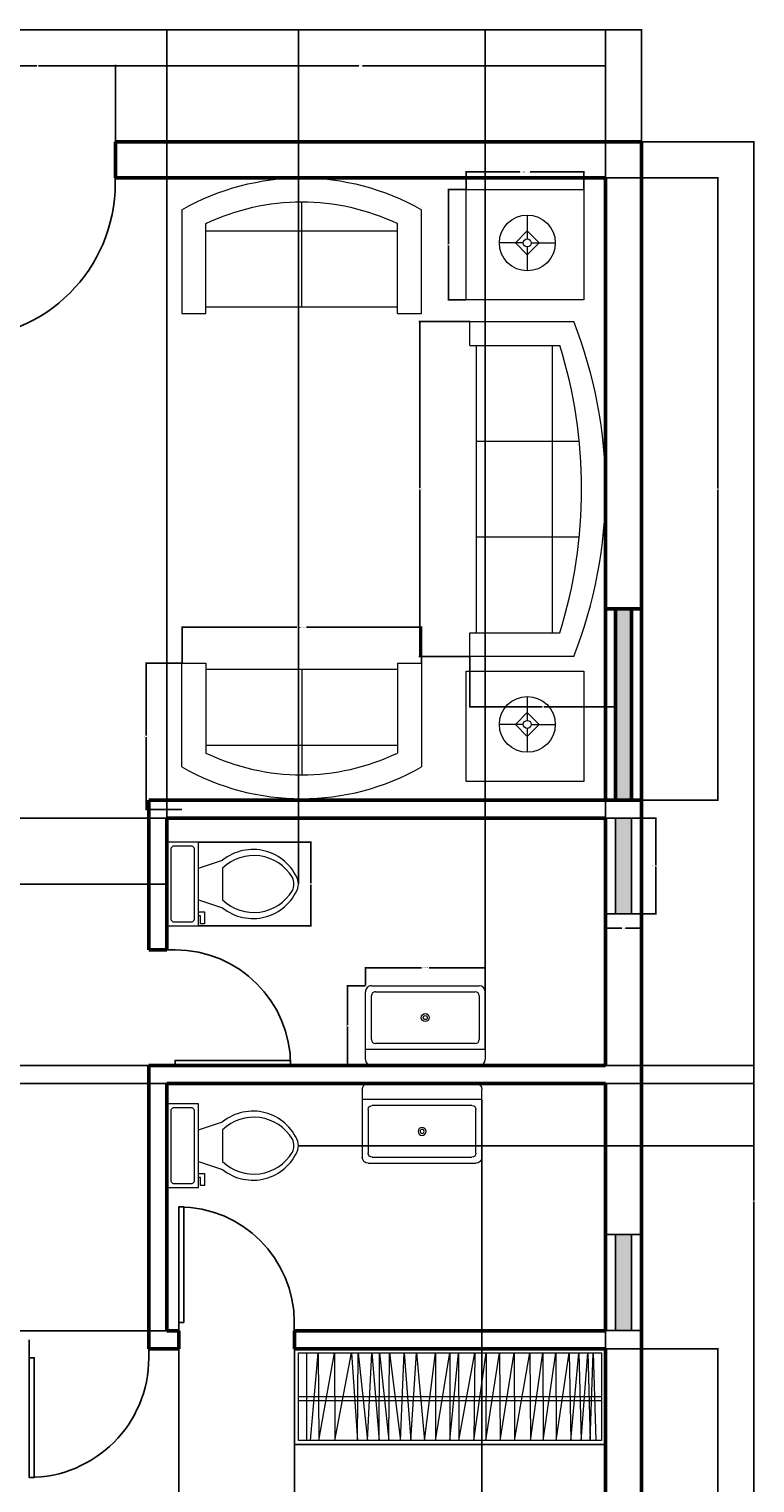
# Model space of a CAD drawing. Units: inches. Extents: x 1974 to 2406, y 1583 to 2170.
# Tile 6 of 6: x 2224 to 2406, y 1806 to 2170. Entities that reach past the tile are written whole.
import ezdxf

# ---------------------------------------------------------------- set-up
doc = ezdxf.new("R2010")
doc.units = ezdxf.units.IN
for name, color, linetype, lineweight in [('A-ANNO-DIMS', 2, 'Continuous', 18), ('A-FLOR-FIXT', 3, 'Continuous', 18), ('A-FURN', 3, 'Continuous', 18), ('A-GLAZ', 4, 'Continuous', 25), ('door', 60, 'Continuous', 25), ('wall', 240, 'Continuous', 50)]:
    doc.layers.add(name, color=color, linetype=linetype, lineweight=lineweight)
doc.layers.add('A-FLOR-CASE', color=40, linetype='Continuous', lineweight=18, true_color=0xf8d731)
doc.styles.get("Standard").update_dxf_attribs({"font": 'arial.ttf'})
doc.dimstyles.get("Standard").update_dxf_attribs({"dimtxt": 0.18, "dimasz": 0.18, "dimexe": 0.18, "dimexo": 0.0625, "dimgap": 0.09, "dimtad": 0, "dimtih": 1, "dimtoh": 1, "dimdec": 4, "dimzin": 0, "dimdsep": 46, "dimtxsty": 'Standard', "dimcen": 0.09, "dimadec": 0, "dimazin": 0, "dimtfac": 1, "dimtdec": 4, "dimtofl": 0, "dimtmove": 0, "dimatfit": 3, "dimfxl": 1, "dimtolj": 1, "dimtzin": 0, "dimarcsym": 0})

# ---------------------------------------------------------------- blocks, each defined once
blk = doc.blocks.new('*U2')
for p, q in [((0, 0), (0, -6)), ((40, 0), (40, -6))]:
    blk.add_line(p, q)
blk.add_lwpolyline([(0, 0), (0, 40), (1.75, 40), (1.75, 0)], close=True)
blk.add_arc((0, 0), 40, 0, 90)
blk = doc.blocks.new('b')
at = {"layer": 'wall'}
h = blk.add_hatch(color=256, dxfattribs=at)
h.dxf.hatch_style = 1
h.paths.add_polyline_path([(6.5, 0), (2.5, 0), (2.5, -48), (6.5, -48)])
for p, q in [((2.5, 0), (2.5, -48)), ((6.5, 0), (6.5, -48))]:
    blk.add_line(p, q, dxfattribs=at)
blk.add_lwpolyline([(0, -48), (9, -48), (9, 0), (0, 0)], close=True, dxfattribs=at)
blk = doc.blocks.new('*U7')
for p, q in [((9.5, -6), (9.5, -2)), ((-10, -8.5), (-8, -8.5)), ((-10, -9.5), (-10, -8.5)), ((-7, -9.5), (-10, -9.5)), ((-8, -8.5), (-8, -8)), ((-7, -8), (-7, -9.5)), ((-4, -8), (-6, -14)), ((4, -8), (6, -14)), ((4, -14), (-4, -14))]:
    blk.add_line(p, q)
blk.add_lwpolyline([(10.5, -8), (10.5, 0), (-10.5, 0), (-10.5, -8)], close=True)
for points in [[(-9.5, -2), (-9.5, -6)], [(8.5, -1), (-8.5, -1)], [(-8.5, -7), (8.5, -7)]]:
    blk.add_lwpolyline(points)
for centre, radius, start, end in [((-8.62, -1.88), 0.884, 81.8699, 188.1301), ((8.62, -1.88), 0.884, 351.8699, 98.1301), ((-8.62, -6.12), 0.884, 171.8699, 278.1301), ((8.62, -6.12), 0.884, 261.8699, 8.1301), ((3.52, -21.58), 12.17, 141.4691, 247.9714), ((4.2, -21.82), 11.33, 136.3677, 238.9468), ((-3.52, -21.58), 12.17, 292.0284, 38.5307), ((-4.2, -21.82), 11.33, 301.053, 43.6321), ((0, -27.88), 4, 245.7318, 294.2682), ((0, -29), 4, 254.8605, 285.1395)]:
    blk.add_arc(centre, radius, start, end)
blk = doc.blocks.new('Sink-single - 30 in top')
blk.add_line((-15, -3.999996), (15, -3.999996))
for points in [[(-13.5, 0), (13.5, 0)], [(-15, -18.499996), (-15, -1.5)], [(15, -1.5), (15, -18.499996)], [(-13.5, -17.499996), (-13.5, -6.499996)], [(-12.5, -5.499996), (12.5, -5.499996)], [(13.5, -6.499996), (13.5, -17.499996)], [(13.5, -19.999996), (-13.5, -19.999996)], [(12.5, -18.499996), (-12.5, -18.499996)]]:
    blk.add_lwpolyline(points)
for radius in [1, 0.5]:
    blk.add_circle((0, -11.999996), radius)
for centre, radius, start, end in [((-13.5, -1.5), 1.5, 90, 180), ((13.5, -1.5), 1.5, 0, 90), ((-12.5, -6.499996), 1, 90, 180), ((12.5, -6.499996), 1, 0, 90), ((-12.5, -17.499996), 1, 180, 270), ((12.5, -17.499996), 1, 270, 0), ((-13.5, -18.499996), 1.5, 180, 270), ((13.5, -18.499996), 1.5, 270, 0)]:
    blk.add_arc(centre, radius, start, end)
blk = doc.blocks.new('Sofa - Roundback 7 ft.')
for p, q in [((-12.00002, -32.4421), (-12.00003, -6.5971)), ((11.99997, -32.4421), (11.99998, -6.5971)), ((-36.000027, -34), (-36.000027, -11.4696)), ((-35.999844, -13.3819), (35.9998, -13.3819)), ((35.99998, -34), (35.99998, -11.4696)), ((-36.000027, -32.4421), (35.99998, -32.4421))]:
    blk.add_line(p, q)
for points in [[(-36.000027, -34), (-42.000027, -34), (-42.000027, -8)], [(41.99998, -8), (41.99998, -34), (35.99998, -34)]]:
    blk.add_lwpolyline(points)
for centre, radius, start, end in [((0, -114.25), 114.25, 68.43141, 111.5686), ((-0.00001, -127.1968), 121.1968, 72.72033, 107.2797)]:
    blk.add_arc(centre, radius, start, end)
blk = doc.blocks.new('Sofa - Roundback Loveseat 5 ft.')
for p, q in [((0, -32.44198), (0, -5.99998)), ((-24, -33.99998), (-24, -11.46958)), ((-23.9998, -13.38178), (23.99986, -13.38178)), ((24.00004, -33.99998), (24.00004, -11.46958)), ((-24, -32.44198), (24.00004, -32.44198))]:
    blk.add_line(p, q)
for points in [[(-24, -33.99998), (-30, -33.99998), (-30, -7.99998)], [(30.00004, -7.99998), (30.00004, -33.99998), (24.00004, -33.99998)]]:
    blk.add_lwpolyline(points)
for centre, radius, start, end in [((0, -60.24998), 60.24998, 60.13715, 119.8628), ((0, -61.38438), 55.38444, 64.32083, 115.6792)]:
    blk.add_arc(centre, radius, start, end)
blk = doc.blocks.new('Lamp - Table')
for p, q in [((0, 7), (0, 1)), ((-1, 0), (-7, 0)), ((0, 3), (-3, 0)), ((-3, 0), (0, -3)), ((3, 0), (0, 3)), ((0, -3), (3, 0)), ((1, 0), (7, 0)), ((0, -1), (0, -7))]:
    blk.add_line(p, q)
for radius in [7, 1]:
    blk.add_circle((0, 0), radius)
blk = doc.blocks.new('WINDOW-24IN')
h = blk.add_hatch(color=256)
h.dxf.hatch_style = 1
h.paths.add_polyline_path([(6.5, 24), (2.5, 24), (2.5, 0), (6.5, 0)])
for p, q in [((2.5, 24), (2.5, 0)), ((6.5, 24), (6.5, 0))]:
    blk.add_line(p, q)
blk.add_lwpolyline([(0, 0), (0, 24), (9, 24), (9, 0)], close=True)
blk = doc.blocks.new('CLOSET-HANGER-RUN')
for p, q in [((0, 0), (0, 22)), ((0.94, 0), (2.86, 22)), ((2.86, 22), (2.99, 0)), ((2.99, 0), (6.93, 22)), ((6.93, 22), (6.99, 0)), ((6.99, 0), (11.19, 22)), ((11.19, 22), (12.71, 0)), ((12.71, 0), (12.83, 22)), ((12.83, 22), (15.2, 0)), ((15.2, 0), (16.24, 22)), ((16.24, 22), (18.1, 0)), ((18.1, 0), (18.16, 22)), ((18.16, 22), (20.55, 0)), ((20.55, 0), (20.68, 22)), ((20.68, 22), (23.44, 0)), ((23.44, 0), (24.36, 22)), ((24.36, 22), (26.08, 0)), ((26.08, 0), (27.44, 22)), ((27.44, 22), (29.52, 0)), ((29.52, 0), (32.2, 22)), ((32.2, 22), (32.2, 0)), ((32.2, 0), (35.87, 22)), ((35.87, 22), (35.87, 0)), ((35.87, 0), (38.02, 22)), ((38.02, 22), (38.12, 0)), ((38.12, 0), (42.07, 22)), ((42.07, 22), (41.87, 0)), ((41.87, 0), (44.93, 22)), ((44.93, 22), (44.83, 0)), ((44.83, 0), (48.29, 22)), ((48.29, 22), (48.48, 0)), ((48.48, 0), (51.94, 22)), ((51.94, 22), (52.04, 0)), ((52.04, 0), (55.89, 22)), ((55.89, 22), (56.08, 0)), ((56.08, 0), (59.14, 22)), ((59.14, 22), (59.24, 0)), ((59.24, 0), (62.4, 22)), ((62.4, 22), (62.5, 0)), ((62.5, 0), (65.76, 22)), ((65.76, 22), (66.15, 0)), ((66.15, 0), (68.13, 22)), ((68.13, 22), (68.72, 0)), ((68.72, 0), (70.4, 22)), ((70.4, 22), (70.99, 0)), ((70.99, 0), (71.78, 22)), ((71.78, 22), (72.44, 0))]:
    blk.add_line(p, q)
blk = doc.blocks.new('TABLE-END')
blk.add_lwpolyline([(0, 27.67), (29.53, 27.67), (29.53, 0), (0, 0)], close=True)
blk = doc.blocks.new('*D24')
at = {"layer": 'A-ANNO-DIMS', "color": 0, "lineweight": -2, "transparency": 16777216}
for p, q in [((2377.72, 1972.49), (2381.44, 1972.49)), ((2381.26, 1972.31), (2381.26, 1960.68)), ((2381.26, 1948.67), (2381.26, 1960.31)), ((2377.72, 1948.49), (2381.44, 1948.49))]:
    blk.add_line(p, q, dxfattribs=at)
at = {"layer": 'A-ANNO-DIMS', "color": 0, "transparency": 16777216}
for points in [[(2381.23, 1972.31), (2381.29, 1972.31), (2381.26, 1972.49)], [(2381.23, 1948.67), (2381.29, 1948.67), (2381.26, 1948.49)]]:
    blk.add_solid(points, dxfattribs=at)
at = {"layer": 'Defpoints', "color": 0, "transparency": 16777216}
for p in [(2377.66, 1972.49), (2381.26, 1972.49), (2377.66, 1948.49)]:
    blk.add_point(p, dxfattribs=at)
at = {"layer": 'A-ANNO-DIMS', "color": 0, "transparency": 16777216, "insert": (2381.26, 1960.49), "char_height": 0.18, "attachment_point": 5}
blk.add_mtext('\\A1;WINDOW 24 TYP.', dxfattribs=at)
blk = doc.blocks.new('*D25')
at = {"layer": 'A-ANNO-DIMS', "color": 0, "lineweight": -2, "transparency": 16777216}
for p, q in [((2368.66, 1948.43), (2368.66, 1944.71)), ((2377.66, 1948.43), (2377.66, 1944.71)), ((2368.84, 1944.89), (2372.7, 1944.89)), ((2377.48, 1944.89), (2373.62, 1944.89))]:
    blk.add_line(p, q, dxfattribs=at)
at = {"layer": 'A-ANNO-DIMS', "color": 0, "transparency": 16777216}
for points in [[(2368.84, 1944.92), (2368.84, 1944.86), (2368.66, 1944.89)], [(2377.48, 1944.92), (2377.48, 1944.86), (2377.66, 1944.89)]]:
    blk.add_solid(points, dxfattribs=at)
at = {"layer": 'Defpoints', "color": 0, "transparency": 16777216}
for p in [(2368.66, 1948.49), (2377.66, 1948.49), (2377.66, 1944.89)]:
    blk.add_point(p, dxfattribs=at)
at = {"layer": 'A-ANNO-DIMS', "color": 0, "transparency": 16777216, "insert": (2373.16, 1944.89), "char_height": 0.18, "attachment_point": 5}
blk.add_mtext('\\A1;9 TYP.', dxfattribs=at)
blk = doc.blocks.new('*D26')
at = {"layer": 'A-ANNO-DIMS', "color": 0, "lineweight": -2, "transparency": 16777216}
for p, q in [((2308.47, 1930.55), (2308.47, 1935.17)), ((2338.47, 1930.55), (2338.47, 1935.17)), ((2308.65, 1934.99), (2322.53, 1934.99)), ((2338.29, 1934.99), (2324.41, 1934.99))]:
    blk.add_line(p, q, dxfattribs=at)
at = {"layer": 'A-ANNO-DIMS', "color": 0, "transparency": 16777216}
for points in [[(2308.65, 1935.02), (2308.65, 1934.96), (2308.47, 1934.99)], [(2338.29, 1935.02), (2338.29, 1934.96), (2338.47, 1934.99)]]:
    blk.add_solid(points, dxfattribs=at)
at = {"layer": 'Defpoints', "color": 0, "transparency": 16777216}
for p in [(2308.47, 1934.99), (2308.47, 1930.49), (2338.47, 1930.49)]:
    blk.add_point(p, dxfattribs=at)
at = {"layer": 'A-ANNO-DIMS', "color": 0, "transparency": 16777216, "insert": (2323.47, 1934.99), "char_height": 0.18, "attachment_point": 5}
blk.add_mtext('\\A1;BASIN 30 TYP.', dxfattribs=at)
blk = doc.blocks.new('*D27')
at = {"layer": 'A-ANNO-DIMS', "color": 0, "lineweight": -2, "transparency": 16777216}
for p, q in [((2308.41, 1930.49), (2303.79, 1930.49)), ((2303.97, 1930.31), (2303.97, 1920.67)), ((2303.97, 1910.67), (2303.97, 1920.31)), ((2308.41, 1910.49), (2303.79, 1910.49))]:
    blk.add_line(p, q, dxfattribs=at)
at = {"layer": 'A-ANNO-DIMS', "color": 0, "transparency": 16777216}
for points in [[(2303.94, 1930.31), (2304, 1930.31), (2303.97, 1930.49)], [(2303.94, 1910.67), (2304, 1910.67), (2303.97, 1910.49)]]:
    blk.add_solid(points, dxfattribs=at)
at = {"layer": 'Defpoints', "color": 0, "transparency": 16777216}
for p in [(2308.47, 1930.49), (2303.97, 1910.49), (2308.47, 1910.49)]:
    blk.add_point(p, dxfattribs=at)
at = {"layer": 'A-ANNO-DIMS', "color": 0, "transparency": 16777216, "insert": (2303.97, 1920.49), "char_height": 0.18, "attachment_point": 5}
blk.add_mtext('\\A1;20 TYP.', dxfattribs=at)
blk = doc.blocks.new('*D34')
at = {"layer": 'A-ANNO-DIMS', "color": 0, "lineweight": -2, "transparency": 16777216}
for p, q in [((2262.49, 2011.42), (2262.49, 2020.54)), ((2262.67, 2020.36), (2291.26, 2020.36)), ((2322.31, 2020.36), (2293.71, 2020.36)), ((2322.49, 2011.42), (2322.49, 2020.54))]:
    blk.add_line(p, q, dxfattribs=at)
at = {"layer": 'A-ANNO-DIMS', "color": 0, "transparency": 16777216}
for points in [[(2262.67, 2020.39), (2262.67, 2020.33), (2262.49, 2020.36)], [(2322.31, 2020.39), (2322.31, 2020.33), (2322.49, 2020.36)]]:
    blk.add_solid(points, dxfattribs=at)
at = {"layer": 'Defpoints', "color": 0, "transparency": 16777216}
for p in [(2262.49, 2020.36), (2262.49, 2011.36), (2322.49, 2011.36)]:
    blk.add_point(p, dxfattribs=at)
at = {"layer": 'A-ANNO-DIMS', "color": 0, "transparency": 16777216, "insert": (2292.49, 2020.36), "char_height": 0.18, "attachment_point": 5}
blk.add_mtext('\\A1;LOVESEAT 60 TYP.', dxfattribs=at)
blk = doc.blocks.new('*D35')
at = {"layer": 'A-ANNO-DIMS', "color": 0, "lineweight": -2, "transparency": 16777216}
for p, q in [((2262.42, 2011.36), (2253.31, 2011.36)), ((2253.49, 2011.18), (2253.49, 1993.2)), ((2253.49, 1974.87), (2253.49, 1992.84)), ((2262.42, 1974.69), (2253.31, 1974.69))]:
    blk.add_line(p, q, dxfattribs=at)
at = {"layer": 'A-ANNO-DIMS', "color": 0, "transparency": 16777216}
for points in [[(2253.46, 2011.18), (2253.52, 2011.18), (2253.49, 2011.36)], [(2253.46, 1974.87), (2253.52, 1974.87), (2253.49, 1974.69)]]:
    blk.add_solid(points, dxfattribs=at)
at = {"layer": 'Defpoints', "color": 0, "transparency": 16777216}
for p in [(2262.49, 2011.36), (2253.49, 1974.69), (2262.49, 1974.69)]:
    blk.add_point(p, dxfattribs=at)
at = {"layer": 'A-ANNO-DIMS', "color": 0, "transparency": 16777216, "insert": (2253.49, 1993.02), "char_height": 0.18, "attachment_point": 5}
blk.add_mtext('\\A1;37 TYP.', dxfattribs=at)
blk = doc.blocks.new('*D36')
at = {"layer": 'A-ANNO-DIMS', "color": 0, "lineweight": -2, "transparency": 16777216}
for p, q in [((2333.69, 2130.13), (2333.69, 2134.67)), ((2333.87, 2134.49), (2347.19, 2134.49)), ((2363.03, 2134.49), (2349.71, 2134.49)), ((2363.21, 2130.13), (2363.21, 2134.67))]:
    blk.add_line(p, q, dxfattribs=at)
at = {"layer": 'A-ANNO-DIMS', "color": 0, "transparency": 16777216}
for points in [[(2333.87, 2134.52), (2333.87, 2134.46), (2333.69, 2134.49)], [(2363.03, 2134.52), (2363.03, 2134.46), (2363.21, 2134.49)]]:
    blk.add_solid(points, dxfattribs=at)
at = {"layer": 'Defpoints', "color": 0, "transparency": 16777216}
for p in [(2363.21, 2134.49), (2333.69, 2130.06), (2363.21, 2130.06)]:
    blk.add_point(p, dxfattribs=at)
at = {"layer": 'A-ANNO-DIMS', "color": 0, "transparency": 16777216, "insert": (2348.45, 2134.49), "char_height": 0.18, "attachment_point": 5}
blk.add_mtext('\\A1;END TABLE 30 TYP.', dxfattribs=at)
blk = doc.blocks.new('*D37')
at = {"layer": 'A-ANNO-DIMS', "color": 0, "lineweight": -2, "transparency": 16777216}
for p, q in [((2333.63, 2130.06), (2329.08, 2130.06)), ((2329.26, 2129.88), (2329.26, 2116.41)), ((2329.26, 2102.57), (2329.26, 2116.05)), ((2333.63, 2102.39), (2329.08, 2102.39))]:
    blk.add_line(p, q, dxfattribs=at)
at = {"layer": 'A-ANNO-DIMS', "color": 0, "transparency": 16777216}
for points in [[(2329.23, 2129.88), (2329.29, 2129.88), (2329.26, 2130.06)], [(2329.23, 2102.57), (2329.29, 2102.57), (2329.26, 2102.39)]]:
    blk.add_solid(points, dxfattribs=at)
at = {"layer": 'Defpoints', "color": 0, "transparency": 16777216}
for p in [(2329.26, 2130.06), (2333.69, 2130.06), (2333.69, 2102.39)]:
    blk.add_point(p, dxfattribs=at)
at = {"layer": 'A-ANNO-DIMS', "color": 0, "transparency": 16777216, "insert": (2329.26, 2116.23), "char_height": 0.18, "attachment_point": 5}
blk.add_mtext('\\A1;28 TYP.', dxfattribs=at)
blk = doc.blocks.new('*D44')
at = {"layer": 'A-ANNO-DIMS', "color": 0, "lineweight": -2, "transparency": 16777216}
for p, q in [((2334.6, 2096.99), (2321.88, 2096.99)), ((2322.06, 2096.81), (2322.06, 2055.18)), ((2322.06, 2013.17), (2322.06, 2054.81)), ((2334.6, 2012.99), (2321.88, 2012.99))]:
    blk.add_line(p, q, dxfattribs=at)
at = {"layer": 'A-ANNO-DIMS', "color": 0, "transparency": 16777216}
for points in [[(2322.03, 2096.81), (2322.09, 2096.81), (2322.06, 2096.99)], [(2322.03, 2013.17), (2322.09, 2013.17), (2322.06, 2012.99)]]:
    blk.add_solid(points, dxfattribs=at)
at = {"layer": 'Defpoints', "color": 0, "transparency": 16777216}
for p in [(2334.66, 2096.99), (2322.06, 2012.99), (2334.66, 2012.99)]:
    blk.add_point(p, dxfattribs=at)
at = {"layer": 'A-ANNO-DIMS', "color": 0, "transparency": 16777216, "insert": (2322.06, 2054.99), "char_height": 0.18, "attachment_point": 5}
blk.add_mtext('\\A1;SOFA 84', dxfattribs=at)
blk = doc.blocks.new('*D45')
at = {"layer": 'A-ANNO-DIMS', "color": 0, "lineweight": -2, "transparency": 16777216}
for p, q in [((2334.66, 2012.93), (2334.66, 2000.21)), ((2371.32, 2012.93), (2371.32, 2000.21)), ((2334.84, 2000.39), (2352.77, 2000.39)), ((2371.14, 2000.39), (2353.21, 2000.39))]:
    blk.add_line(p, q, dxfattribs=at)
at = {"layer": 'A-ANNO-DIMS', "color": 0, "transparency": 16777216}
for points in [[(2334.84, 2000.42), (2334.84, 2000.36), (2334.66, 2000.39)], [(2371.14, 2000.42), (2371.14, 2000.36), (2371.32, 2000.39)]]:
    blk.add_solid(points, dxfattribs=at)
at = {"layer": 'Defpoints', "color": 0, "transparency": 16777216}
for p in [(2334.66, 2012.99), (2371.32, 2012.99), (2371.32, 2000.39)]:
    blk.add_point(p, dxfattribs=at)
at = {"layer": 'A-ANNO-DIMS', "color": 0, "transparency": 16777216, "insert": (2352.99, 2000.39), "char_height": 0.18, "attachment_point": 5}
blk.add_mtext('\\A1;37', dxfattribs=at)
blk = doc.blocks.new('*D48')
at = {"layer": 'A-ANNO-DIMS', "color": 0, "lineweight": -2, "transparency": 16777216}
for p, q in [((2002.16, 2142.05), (2002.16, 2170.29)), ((2002.34, 2170.11), (2189.51, 2170.11)), ((2377.48, 2170.11), (2190.3, 2170.11)), ((2377.66, 2142.05), (2377.66, 2170.29))]:
    blk.add_line(p, q, dxfattribs=at)
at = {"layer": 'A-ANNO-DIMS', "color": 0, "transparency": 16777216}
for points in [[(2002.34, 2170.14), (2002.34, 2170.08), (2002.16, 2170.11)], [(2377.48, 2170.14), (2377.48, 2170.08), (2377.66, 2170.11)]]:
    blk.add_solid(points, dxfattribs=at)
at = {"layer": 'Defpoints', "color": 0, "transparency": 16777216}
for p in [(2377.66, 2170.11), (2002.16, 2141.99), (2377.66, 2141.99)]:
    blk.add_point(p, dxfattribs=at)
at = {"layer": 'A-ANNO-DIMS', "color": 0, "transparency": 16777216, "insert": (2189.91, 2170.11), "char_height": 0.18, "attachment_point": 5}
blk.add_mtext('\\A1;375.5', dxfattribs=at)
blk = doc.blocks.new('*D49')
at = {"layer": 'A-ANNO-DIMS', "color": 0, "lineweight": -2, "transparency": 16777216}
for p, q in [((2377.72, 2141.99), (2405.96, 2141.99)), ((2405.78, 2141.81), (2405.78, 1876.67)), ((2405.78, 1611.17), (2405.78, 1876.31)), ((2377.72, 1610.99), (2405.96, 1610.99))]:
    blk.add_line(p, q, dxfattribs=at)
at = {"layer": 'A-ANNO-DIMS', "color": 0, "transparency": 16777216}
for points in [[(2405.75, 2141.81), (2405.81, 2141.81), (2405.78, 2141.99)], [(2405.75, 1611.17), (2405.81, 1611.17), (2405.78, 1610.99)]]:
    blk.add_solid(points, dxfattribs=at)
at = {"layer": 'Defpoints', "color": 0, "transparency": 16777216}
for p in [(2377.66, 2141.99), (2377.66, 1610.99), (2405.78, 1610.99)]:
    blk.add_point(p, dxfattribs=at)
at = {"layer": 'A-ANNO-DIMS', "color": 0, "transparency": 16777216, "insert": (2405.78, 1876.49), "char_height": 0.18, "attachment_point": 5}
blk.add_mtext('\\A1;531', dxfattribs=at)
blk = doc.blocks.new('*D52')
at = {"layer": 'A-ANNO-DIMS', "color": 0, "lineweight": -2, "transparency": 16777216}
for p, q in [((2206.82, 2133.05), (2206.82, 2161.29)), ((2207, 2161.11), (2226.1, 2161.11)), ((2245.64, 2161.11), (2226.54, 2161.11)), ((2245.82, 2133.05), (2245.82, 2161.29))]:
    blk.add_line(p, q, dxfattribs=at)
at = {"layer": 'A-ANNO-DIMS', "color": 0, "transparency": 16777216}
for points in [[(2207, 2161.14), (2207, 2161.08), (2206.82, 2161.11)], [(2245.64, 2161.14), (2245.64, 2161.08), (2245.82, 2161.11)]]:
    blk.add_solid(points, dxfattribs=at)
at = {"layer": 'Defpoints', "color": 0, "transparency": 16777216}
for p in [(2245.82, 2161.11), (2206.82, 2132.99), (2245.82, 2132.99)]:
    blk.add_point(p, dxfattribs=at)
at = {"layer": 'A-ANNO-DIMS', "color": 0, "transparency": 16777216, "insert": (2226.32, 2161.11), "char_height": 0.18, "attachment_point": 5}
blk.add_mtext('\\A1;39', dxfattribs=at)
blk = doc.blocks.new('*D53')
at = {"layer": 'A-ANNO-DIMS', "color": 0, "lineweight": -2, "transparency": 16777216}
for p, q in [((2245.82, 2133.05), (2245.82, 2161.29)), ((2246, 2161.11), (2306.78, 2161.11)), ((2368.48, 2161.11), (2307.69, 2161.11)), ((2368.66, 2133.05), (2368.66, 2161.29))]:
    blk.add_line(p, q, dxfattribs=at)
at = {"layer": 'A-ANNO-DIMS', "color": 0, "transparency": 16777216}
for points in [[(2246, 2161.14), (2246, 2161.08), (2245.82, 2161.11)], [(2368.48, 2161.14), (2368.48, 2161.08), (2368.66, 2161.11)]]:
    blk.add_solid(points, dxfattribs=at)
at = {"layer": 'Defpoints', "color": 0, "transparency": 16777216}
for p in [(2368.66, 2161.11), (2245.82, 2132.99), (2368.66, 2132.99)]:
    blk.add_point(p, dxfattribs=at)
at = {"layer": 'A-ANNO-DIMS', "color": 0, "transparency": 16777216, "insert": (2307.24, 2161.11), "char_height": 0.18, "attachment_point": 5}
blk.add_mtext('\\A1;122.84', dxfattribs=at)
blk = doc.blocks.new('*D59')
at = {"layer": 'A-ANNO-DIMS', "color": 0, "lineweight": -2, "transparency": 16777216}
for p, q in [((2368.72, 2132.99), (2396.96, 2132.99)), ((2396.78, 2132.81), (2396.78, 2055.17)), ((2396.78, 1977.17), (2396.78, 2054.81)), ((2368.72, 1976.99), (2396.96, 1976.99))]:
    blk.add_line(p, q, dxfattribs=at)
at = {"layer": 'A-ANNO-DIMS', "color": 0, "transparency": 16777216}
for points in [[(2396.75, 2132.81), (2396.81, 2132.81), (2396.78, 2132.99)], [(2396.75, 1977.17), (2396.81, 1977.17), (2396.78, 1976.99)]]:
    blk.add_solid(points, dxfattribs=at)
at = {"layer": 'Defpoints', "color": 0, "transparency": 16777216}
for p in [(2368.66, 2132.99), (2368.66, 1976.99), (2396.78, 1976.99)]:
    blk.add_point(p, dxfattribs=at)
at = {"layer": 'A-ANNO-DIMS', "color": 0, "transparency": 16777216, "insert": (2396.78, 2054.99), "char_height": 0.18, "attachment_point": 5}
blk.add_mtext('\\A1;156', dxfattribs=at)
blk = doc.blocks.new('*D60')
at = {"layer": 'A-ANNO-DIMS', "color": 0, "lineweight": -2, "transparency": 16777216}
for p, q in [((2368.72, 1839.49), (2396.96, 1839.49)), ((2396.78, 1839.31), (2396.78, 1771.92)), ((2396.78, 1704.17), (2396.78, 1771.56)), ((2368.72, 1703.99), (2396.96, 1703.99))]:
    blk.add_line(p, q, dxfattribs=at)
at = {"layer": 'A-ANNO-DIMS', "color": 0, "transparency": 16777216}
for points in [[(2396.75, 1839.31), (2396.81, 1839.31), (2396.78, 1839.49)], [(2396.75, 1704.17), (2396.81, 1704.17), (2396.78, 1703.99)]]:
    blk.add_solid(points, dxfattribs=at)
at = {"layer": 'Defpoints', "color": 0, "transparency": 16777216}
for p in [(2368.66, 1839.49), (2368.66, 1703.99), (2396.78, 1703.99)]:
    blk.add_point(p, dxfattribs=at)
at = {"layer": 'A-ANNO-DIMS', "color": 0, "transparency": 16777216, "insert": (2396.78, 1771.74), "char_height": 0.18, "attachment_point": 5}
blk.add_mtext('\\A1;135.5', dxfattribs=at)
blk = doc.blocks.new('*D72')
at = {"layer": 'A-ANNO-DIMS', "color": 0, "lineweight": -2, "transparency": 16777216}
for p, q in [((2258.66, 1972.55), (2258.66, 2170.29)), ((2258.84, 2170.11), (2313.38, 2170.11)), ((2368.48, 2170.11), (2313.94, 2170.11)), ((2368.66, 1972.55), (2368.66, 2170.29))]:
    blk.add_line(p, q, dxfattribs=at)
at = {"layer": 'A-ANNO-DIMS', "color": 0, "transparency": 16777216}
for points in [[(2258.84, 2170.14), (2258.84, 2170.08), (2258.66, 2170.11)], [(2368.48, 2170.14), (2368.48, 2170.08), (2368.66, 2170.11)]]:
    blk.add_solid(points, dxfattribs=at)
at = {"layer": 'Defpoints', "color": 0, "transparency": 16777216}
for p in [(2368.66, 2170.11), (2258.66, 1972.49), (2368.66, 1972.49)]:
    blk.add_point(p, dxfattribs=at)
at = {"layer": 'A-ANNO-DIMS', "color": 0, "transparency": 16777216, "insert": (2313.66, 2170.11), "char_height": 0.18, "attachment_point": 5}
blk.add_mtext('\\A1;110', dxfattribs=at)
blk = doc.blocks.new('*D73')
at = {"layer": 'A-ANNO-DIMS', "color": 0, "lineweight": -2, "transparency": 16777216}
for p, q in [((2258.6, 1972.49), (1973.86, 1972.49)), ((1974.04, 1972.31), (1974.04, 1941.67)), ((1974.04, 1910.67), (1974.04, 1941.31)), ((2254.1, 1910.49), (1973.86, 1910.49))]:
    blk.add_line(p, q, dxfattribs=at)
at = {"layer": 'A-ANNO-DIMS', "color": 0, "transparency": 16777216}
for points in [[(1974.01, 1972.31), (1974.07, 1972.31), (1974.04, 1972.49)], [(1974.01, 1910.67), (1974.07, 1910.67), (1974.04, 1910.49)]]:
    blk.add_solid(points, dxfattribs=at)
at = {"layer": 'Defpoints', "color": 0, "transparency": 16777216}
for p in [(2258.66, 1972.49), (1974.04, 1910.49), (2254.16, 1910.49)]:
    blk.add_point(p, dxfattribs=at)
at = {"layer": 'A-ANNO-DIMS', "color": 0, "transparency": 16777216, "insert": (1974.04, 1941.49), "char_height": 0.18, "attachment_point": 5}
blk.add_mtext('\\A1;62', dxfattribs=at)
blk = doc.blocks.new('*D74')
at = {"layer": 'A-ANNO-DIMS', "color": 0, "lineweight": -2, "transparency": 16777216}
for p, q in [((2368.72, 1910.49), (2405.96, 1910.49)), ((2405.78, 1910.31), (2405.78, 1908.42)), ((2368.72, 1905.99), (2405.96, 1905.99)), ((2405.78, 1906.17), (2405.78, 1908.06))]:
    blk.add_line(p, q, dxfattribs=at)
at = {"layer": 'A-ANNO-DIMS', "color": 0, "transparency": 16777216}
for points in [[(2405.75, 1910.31), (2405.81, 1910.31), (2405.78, 1910.49)], [(2405.75, 1906.17), (2405.81, 1906.17), (2405.78, 1905.99)]]:
    blk.add_solid(points, dxfattribs=at)
at = {"layer": 'Defpoints', "color": 0, "transparency": 16777216}
for p in [(2368.66, 1910.49), (2368.66, 1905.99), (2405.78, 1905.99)]:
    blk.add_point(p, dxfattribs=at)
at = {"layer": 'A-ANNO-DIMS', "color": 0, "transparency": 16777216, "insert": (2405.78, 1908.24), "char_height": 0.18, "attachment_point": 5}
blk.add_mtext('\\A1;4.5', dxfattribs=at)
blk = doc.blocks.new('*D75')
at = {"layer": 'A-ANNO-DIMS', "color": 0, "lineweight": -2, "transparency": 16777216}
for p, q in [((2258.6, 1905.99), (1973.86, 1905.99)), ((1974.04, 1905.81), (1974.04, 1875.17)), ((1974.04, 1844.17), (1974.04, 1874.81)), ((2258.6, 1843.99), (1973.86, 1843.99))]:
    blk.add_line(p, q, dxfattribs=at)
at = {"layer": 'A-ANNO-DIMS', "color": 0, "transparency": 16777216}
for points in [[(1974.01, 1905.81), (1974.07, 1905.81), (1974.04, 1905.99)], [(1974.01, 1844.17), (1974.07, 1844.17), (1974.04, 1843.99)]]:
    blk.add_solid(points, dxfattribs=at)
at = {"layer": 'Defpoints', "color": 0, "transparency": 16777216}
for p in [(2258.66, 1905.99), (1974.04, 1843.99), (2258.66, 1843.99)]:
    blk.add_point(p, dxfattribs=at)
at = {"layer": 'A-ANNO-DIMS', "color": 0, "transparency": 16777216, "insert": (1974.04, 1874.99), "char_height": 0.18, "attachment_point": 5}
blk.add_mtext('\\A1;62', dxfattribs=at)
blk = doc.blocks.new('*D76')
at = {"layer": 'A-ANNO-DIMS', "color": 0, "lineweight": -2, "transparency": 16777216}
for p, q in [((2261.66, 1839.43), (2261.66, 1582.69)), ((2290.66, 1839.43), (2290.66, 1582.69)), ((2261.84, 1582.87), (2275.94, 1582.87)), ((2290.48, 1582.87), (2276.38, 1582.87))]:
    blk.add_line(p, q, dxfattribs=at)
at = {"layer": 'A-ANNO-DIMS', "color": 0, "transparency": 16777216}
for points in [[(2261.84, 1582.9), (2261.84, 1582.84), (2261.66, 1582.87)], [(2290.48, 1582.9), (2290.48, 1582.84), (2290.66, 1582.87)]]:
    blk.add_solid(points, dxfattribs=at)
at = {"layer": 'Defpoints', "color": 0, "transparency": 16777216}
for p in [(2261.66, 1839.49), (2290.66, 1839.49), (2290.66, 1582.87)]:
    blk.add_point(p, dxfattribs=at)
at = {"layer": 'A-ANNO-DIMS', "color": 0, "transparency": 16777216, "insert": (2276.16, 1582.87), "char_height": 0.18, "attachment_point": 5}
blk.add_mtext('\\A1;29', dxfattribs=at)
blk = doc.blocks.new('*D77')
at = {"layer": 'A-ANNO-DIMS', "color": 0, "lineweight": -2, "transparency": 16777216}
for p, q in [((2258.66, 1966.55), (2258.66, 2170.29)), ((2258.84, 2170.11), (2274.94, 2170.11)), ((2291.48, 2170.11), (2275.38, 2170.11)), ((2291.66, 1956.05), (2291.66, 2170.29))]:
    blk.add_line(p, q, dxfattribs=at)
at = {"layer": 'A-ANNO-DIMS', "color": 0, "transparency": 16777216}
for points in [[(2258.84, 2170.14), (2258.84, 2170.08), (2258.66, 2170.11)], [(2291.48, 2170.14), (2291.48, 2170.08), (2291.66, 2170.11)]]:
    blk.add_solid(points, dxfattribs=at)
at = {"layer": 'Defpoints', "color": 0, "transparency": 16777216}
for p in [(2291.66, 2170.11), (2258.66, 1966.49), (2291.66, 1955.99)]:
    blk.add_point(p, dxfattribs=at)
at = {"layer": 'A-ANNO-DIMS', "color": 0, "transparency": 16777216, "insert": (2275.16, 2170.11), "char_height": 0.18, "attachment_point": 5}
blk.add_mtext('\\A1;33', dxfattribs=at)
blk = doc.blocks.new('*D78')
at = {"layer": 'A-ANNO-DIMS', "color": 0, "lineweight": -2, "transparency": 16777216}
for p, q in [((2266.72, 1966.49), (2294.96, 1966.49)), ((2294.78, 1966.31), (2294.78, 1956.17)), ((2294.78, 1945.67), (2294.78, 1955.81)), ((2266.72, 1945.49), (2294.96, 1945.49))]:
    blk.add_line(p, q, dxfattribs=at)
at = {"layer": 'A-ANNO-DIMS', "color": 0, "transparency": 16777216}
for points in [[(2294.75, 1966.31), (2294.81, 1966.31), (2294.78, 1966.49)], [(2294.75, 1945.67), (2294.81, 1945.67), (2294.78, 1945.49)]]:
    blk.add_solid(points, dxfattribs=at)
at = {"layer": 'Defpoints', "color": 0, "transparency": 16777216}
for p in [(2266.66, 1966.49), (2266.66, 1945.49), (2294.78, 1945.49)]:
    blk.add_point(p, dxfattribs=at)
at = {"layer": 'A-ANNO-DIMS', "color": 0, "transparency": 16777216, "insert": (2294.78, 1955.99), "char_height": 0.18, "attachment_point": 5}
blk.add_mtext('\\A1;21', dxfattribs=at)
blk = doc.blocks.new('*D79')
at = {"layer": 'A-ANNO-DIMS', "color": 0, "lineweight": -2, "transparency": 16777216}
for p, q in [((2368.66, 1905.93), (2368.66, 1582.69)), ((2337.66, 1901.93), (2337.66, 1582.69)), ((2337.84, 1582.87), (2352.7, 1582.87)), ((2368.48, 1582.87), (2353.62, 1582.87))]:
    blk.add_line(p, q, dxfattribs=at)
at = {"layer": 'A-ANNO-DIMS', "color": 0, "transparency": 16777216}
for points in [[(2337.84, 1582.9), (2337.84, 1582.84), (2337.66, 1582.87)], [(2368.48, 1582.9), (2368.48, 1582.84), (2368.66, 1582.87)]]:
    blk.add_solid(points, dxfattribs=at)
at = {"layer": 'Defpoints', "color": 0, "transparency": 16777216}
for p in [(2368.66, 1905.99), (2337.66, 1901.99), (2368.66, 1582.87)]:
    blk.add_point(p, dxfattribs=at)
at = {"layer": 'A-ANNO-DIMS', "color": 0, "transparency": 16777216, "insert": (2353.16, 1582.87), "char_height": 0.18, "attachment_point": 5}
blk.add_mtext('\\A1;30.994', dxfattribs=at)
blk = doc.blocks.new('*D80')
at = {"layer": 'A-ANNO-DIMS', "color": 0, "lineweight": -2, "transparency": 16777216}
for p, q in [((2338.47, 1914.55), (2338.47, 2170.29)), ((2338.65, 2170.11), (2353.17, 2170.11)), ((2368.48, 2170.11), (2353.96, 2170.11)), ((2368.66, 1910.55), (2368.66, 2170.29))]:
    blk.add_line(p, q, dxfattribs=at)
at = {"layer": 'A-ANNO-DIMS', "color": 0, "transparency": 16777216}
for points in [[(2338.65, 2170.14), (2338.65, 2170.08), (2338.47, 2170.11)], [(2368.48, 2170.14), (2368.48, 2170.08), (2368.66, 2170.11)]]:
    blk.add_solid(points, dxfattribs=at)
at = {"layer": 'Defpoints', "color": 0, "transparency": 16777216}
for p in [(2368.66, 2170.11), (2338.47, 1914.49), (2368.66, 1910.49)]:
    blk.add_point(p, dxfattribs=at)
at = {"layer": 'A-ANNO-DIMS', "color": 0, "transparency": 16777216, "insert": (2353.56, 2170.11), "char_height": 0.18, "attachment_point": 5}
blk.add_mtext('\\A1;30.19', dxfattribs=at)
blk = doc.blocks.new('*D81')
at = {"layer": 'A-ANNO-DIMS', "color": 0, "lineweight": -2, "transparency": 16777216}
for p, q in [((2258.6, 1972.49), (1973.86, 1972.49)), ((1974.04, 1972.31), (1974.04, 1964.42)), ((1974.04, 1956.17), (1974.04, 1964.06)), ((2258.6, 1955.99), (1973.86, 1955.99))]:
    blk.add_line(p, q, dxfattribs=at)
at = {"layer": 'A-ANNO-DIMS', "color": 0, "transparency": 16777216}
for points in [[(1974.01, 1972.31), (1974.07, 1972.31), (1974.04, 1972.49)], [(1974.01, 1956.17), (1974.07, 1956.17), (1974.04, 1955.99)]]:
    blk.add_solid(points, dxfattribs=at)
at = {"layer": 'Defpoints', "color": 0, "transparency": 16777216}
for p in [(1974.04, 1972.49), (2258.66, 1972.49), (2258.66, 1955.99)]:
    blk.add_point(p, dxfattribs=at)
at = {"layer": 'A-ANNO-DIMS', "color": 0, "transparency": 16777216, "insert": (1974.04, 1964.24), "char_height": 0.18, "attachment_point": 5}
blk.add_mtext('\\A1;16.5', dxfattribs=at)
blk = doc.blocks.new('*D82')
at = {"layer": 'A-ANNO-DIMS', "color": 0, "lineweight": -2, "transparency": 16777216}
for p, q in [((2258.72, 1905.99), (2405.96, 1905.99)), ((2405.78, 1905.81), (2405.78, 1898.38)), ((2405.78, 1890.58), (2405.78, 1898.01)), ((2291.72, 1890.4), (2405.96, 1890.4))]:
    blk.add_line(p, q, dxfattribs=at)
at = {"layer": 'A-ANNO-DIMS', "color": 0, "transparency": 16777216}
for points in [[(2405.75, 1905.81), (2405.81, 1905.81), (2405.78, 1905.99)], [(2405.75, 1890.58), (2405.81, 1890.58), (2405.78, 1890.4)]]:
    blk.add_solid(points, dxfattribs=at)
at = {"layer": 'Defpoints', "color": 0, "transparency": 16777216}
for p in [(2258.66, 1905.99), (2405.78, 1905.99), (2291.66, 1890.4)]:
    blk.add_point(p, dxfattribs=at)
at = {"layer": 'A-ANNO-DIMS', "color": 0, "transparency": 16777216, "insert": (2405.78, 1898.2), "char_height": 0.18, "attachment_point": 5}
blk.add_mtext('\\A1;15.59', dxfattribs=at)

msp = doc.modelspace()

# ---------------------------------------------------------------- linework, layer by layer
at = {"layer": 'A-FLOR-CASE'}
for p, q in [((2290.6581, 1839.4921), (2290.6581, 1815.4921)), ((2291.6581, 1827.4921), (2367.6581, 1827.4921)), ((2291.6581, 1826.4921), (2367.6581, 1826.4921)), ((2290.6581, 1815.4921), (2368.6581, 1815.4921))]:
    msp.add_line(p, q, dxfattribs=at)
for points in [[(2290.6581, 1839.4921), (2368.6581, 1839.4921), (2368.6581, 1815.4921), (2290.6581, 1815.4921)], [(2291.6581, 1838.4921), (2367.6581, 1838.4921), (2367.6581, 1816.4921), (2291.6581, 1816.4921)]]:
    msp.add_lwpolyline(points, close=True, dxfattribs=at)
at = {"layer": 'wall'}
for p, q in [((2245.8193, 2132.9921), (2245.8193, 2141.9921)), ((2245.8193, 2141.9921), (2377.6581, 2141.9921)), ((2377.6581, 2141.9921), (2377.6581, 1976.9921)), ((2377.6581, 2141.9921), (2377.6581, 1610.9921)), ((2245.8193, 2132.9921), (2368.6581, 2132.9921)), ((2368.6581, 2132.9921), (2368.6581, 1976.9921)), ((2368.6581, 2132.9921), (2368.6581, 1976.9921)), ((2254.1581, 1976.9921), (2368.6581, 1976.9921)), ((2254.1581, 1976.9921), (2254.1581, 1939.4921)), ((2258.6581, 1972.4921), (2368.6581, 1972.4921)), ((2258.6581, 1972.4921), (2258.6581, 1939.4921)), ((2368.6581, 1972.4921), (2368.6581, 1910.4921)), ((2258.6581, 1939.4921), (2254.1581, 1939.4921)), ((2258.6581, 1910.4921), (2254.1581, 1910.4921)), ((2254.1581, 1910.4921), (2254.1581, 1843.9921)), ((2258.6581, 1910.4921), (2368.6581, 1910.4921)), ((2258.6581, 1905.9921), (2368.6581, 1905.9921)), ((2258.6581, 1905.9921), (2258.6581, 1843.9921)), ((2368.6581, 1905.9921), (2368.6581, 1843.9921)), ((2254.1685, 1839.4921), (2254.1581, 1843.9921)), ((2258.6581, 1843.9921), (2261.6581, 1843.9921)), ((2258.6581, 1843.9921), (2261.6581, 1843.9921)), ((2261.6581, 1843.9921), (2261.6581, 1839.4921)), ((2290.6581, 1843.9921), (2290.6581, 1839.4921)), ((2290.6581, 1843.9921), (2368.6581, 1843.9921)), ((2254.1685, 1839.4921), (2261.6581, 1839.4921)), ((2290.6581, 1839.4921), (2368.6581, 1839.4921)), ((2368.6581, 1839.4921), (2368.6581, 1703.9921))]:
    msp.add_line(p, q, dxfattribs=at)

# ---------------------------------------------------------------- block references
at = {"layer": 'A-FLOR-CASE'}
msp.add_blockref('CLOSET-HANGER-RUN', (2293.788, 1816.492), dxfattribs=at)
at = {"layer": 'A-FLOR-FIXT'}
for name, p, rotation in [('*U7', (2258.6581, 1955.9921), 90), ('Sink-single - 30 in top', (2323.4704, 1910.4921), 180), ('*U7', (2258.6581, 1890.4013), 90)]:
    msp.add_blockref(name, p, dxfattribs=dict(at, rotation=rotation))
at = {"layer": 'A-FLOR-FIXT', "xscale": -1}
msp.add_blockref('Sink-single - 30 in top', (2322.6638, 1905.9921), dxfattribs=at)
at = {"layer": 'A-FURN', "xscale": -1}
msp.add_blockref('Sofa - Roundback Loveseat 5 ft.', (2292.4869, 2132.9921), dxfattribs=at)
at = {"layer": 'A-FURN'}
for name, p in [('TABLE-END', (2333.689, 2102.3927)), ('Lamp - Table', (2349.0343, 2116.6779)), ('TABLE-END', (2333.689, 1981.713)), ('Lamp - Table', (2349.0343, 1995.9982))]:
    msp.add_blockref(name, p, dxfattribs=at)
for name, p, rotation in [('Sofa - Roundback 7 ft.', (2368.6581, 2054.9921), 270), ('Sofa - Roundback Loveseat 5 ft.', (2292.4869, 1977.3556), 180)]:
    msp.add_blockref(name, p, dxfattribs=dict(at, rotation=rotation))
at = {"layer": 'A-GLAZ'}
for name, p in [('b', (2368.6581, 2024.9921)), ('WINDOW-24IN', (2368.658, 1948.492)), ('WINDOW-24IN', (2368.658, 1844.1))]:
    msp.add_blockref(name, p, dxfattribs=at)
at = {"layer": 'door'}
for p, xscale, yscale, zscale, rotation in [((2206.8193, 2131.6526), -0.9732547723877202, 0.9732547723877202, 0.9732547723877202, 180), ((2260.7532, 1910.5245), -0.7241897714673384, 0.7241897714673384, 0.7241897714673384, 270), ((2224.1626, 1837.242), -0.7500157248215027, 0.7500157248215027, 0.7500157248215027, 180)]:
    msp.add_blockref('*U2', p, dxfattribs=dict(at, xscale=xscale, yscale=yscale, zscale=zscale, rotation=rotation))
at = {"layer": 'door', "xscale": 0.7241897714673384, "yscale": 0.7241897714673384, "zscale": 0.7241897714673384}
msp.add_blockref('*U2', (2261.6581, 1846.0872), dxfattribs=at)

# ---------------------------------------------------------------- dimensions: what is measured, and where the dimension line sits
at = {"layer": 'A-ANNO-DIMS'}
for base, p1, p2, override, picture, middle in [((2377.6581, 2170.1096), (2002.1581, 2141.9921), (2377.6581, 2141.9921), {"dimdec": 1, "dimlfac": 1, "dimrnd": 0, "dimzin": 0, "dimdsep": 46, "dimlunit": 2}, '*D48', (2189.9081, 2170.1096)), ((2368.6581, 2170.1096), (2258.6581, 1972.4921), (2368.6581, 1972.4921), {"dimdec": 0, "dimlfac": 1, "dimrnd": 0, "dimzin": 0, "dimdsep": 46, "dimlunit": 2}, '*D72', (2313.6581, 2170.1096)), ((2291.658, 2170.1096), (2258.6581, 1966.4921), (2291.658, 1955.9921), {"dimdec": 0, "dimlfac": 1, "dimrnd": 0, "dimzin": 0, "dimdsep": 46, "dimlunit": 2}, '*D77', (2275.158, 2170.1096)), ((2368.6581, 2170.1096), (2338.4704, 1914.4921), (2368.6581, 1910.4921), {"dimdec": 2, "dimlfac": 1, "dimrnd": 0, "dimzin": 0, "dimdsep": 46, "dimlunit": 2}, '*D80', (2353.5642, 2170.1096)), ((2245.8193, 2161.1096), (2206.8193, 2132.9921), (2245.8193, 2132.9921), {"dimdec": 0, "dimlfac": 1, "dimrnd": 0, "dimzin": 0, "dimdsep": 46, "dimlunit": 2}, '*D52', (2226.3193, 2161.1096)), ((2368.6581, 2161.1096), (2245.8193, 2132.9921), (2368.6581, 2132.9921), {"dimdec": 2, "dimlfac": 1, "dimrnd": 0, "dimzin": 0, "dimdsep": 46, "dimlunit": 2}, '*D53', (2307.2387, 2161.1096)), ((2371.3247, 2000.3921), (2334.6581, 2012.9921), (2371.3247, 2012.9921), {"dimdec": 0, "dimlfac": 1, "dimrnd": 0, "dimzin": 0, "dimdsep": 46, "dimlunit": 2}, '*D45', (2352.9914, 2000.3921)), ((2368.6581, 1582.8746), (2337.6638, 1901.9921), (2368.6581, 1905.9921), {"dimdec": 3, "dimlfac": 1, "dimrnd": 0, "dimzin": 0, "dimdsep": 46, "dimlunit": 2}, '*D79', (2353.1609, 1582.8746)), ((2290.6581, 1582.8746), (2261.6581, 1839.4921), (2290.6581, 1839.4921), {"dimdec": 0, "dimlfac": 1, "dimrnd": 0, "dimzin": 0, "dimdsep": 46, "dimlunit": 2}, '*D76', (2276.1581, 1582.8746))]:
    dim = msp.add_linear_dim(base=base, p1=p1, p2=p2, dimstyle='Standard', override=override, dxfattribs=at)
    dim.commit()
    dim.dimension.update_dxf_attribs({"geometry": picture, "text_midpoint": middle})
for base, p1, p2, angle, override, picture, middle in [((2405.7756, 1610.9921), (2377.6581, 2141.9921), (2377.6581, 1610.9921), 90, {"dimdec": 0, "dimlfac": 1, "dimrnd": 0, "dimzin": 0, "dimdsep": 46, "dimlunit": 2}, '*D49', (2405.7756, 1876.4921)), ((2396.7756, 1976.9921), (2368.6581, 2132.9921), (2368.6581, 1976.9921), 270, {"dimdec": 0, "dimlfac": 1, "dimrnd": 0, "dimzin": 0, "dimdsep": 46, "dimlunit": 2}, '*D59', (2396.7756, 2054.9921)), ((1974.0406, 1972.4921), (2258.6581, 1955.9921), (2258.6581, 1972.4921), 90, {"dimdec": 1, "dimlfac": 1, "dimrnd": 0, "dimzin": 0, "dimdsep": 46, "dimlunit": 2}, '*D81', (1974.0406, 1964.2421)), ((1974.0406, 1910.4921), (2258.6581, 1972.4921), (2254.1581, 1910.4921), 90, {"dimdec": 0, "dimlfac": 1, "dimrnd": 0, "dimzin": 0, "dimdsep": 46, "dimlunit": 2}, '*D73', (1974.0406, 1941.4921)), ((2294.7756, 1945.4921), (2266.6581, 1966.4921), (2266.6581, 1945.4921), 270, {"dimdec": 0, "dimlfac": 1, "dimrnd": 0, "dimzin": 0, "dimdsep": 46, "dimlunit": 2}, '*D78', (2294.7756, 1955.9921)), ((2405.7756, 1905.9921), (2368.6581, 1910.4921), (2368.6581, 1905.9921), 90, {"dimdec": 1, "dimlfac": 1, "dimrnd": 0, "dimzin": 0, "dimdsep": 46, "dimlunit": 2}, '*D74', (2405.7756, 1908.2421)), ((1974.0406, 1843.9921), (2258.6581, 1905.9921), (2258.6581, 1843.9921), 90, {"dimdec": 0, "dimlfac": 1, "dimrnd": 0, "dimzin": 0, "dimdsep": 46, "dimlunit": 2}, '*D75', (1974.0406, 1874.9921)), ((2405.7756, 1905.9921), (2291.658, 1890.4013), (2258.6581, 1905.9921), 90, {"dimdec": 2, "dimlfac": 1, "dimrnd": 0, "dimzin": 0, "dimdsep": 46, "dimlunit": 2}, '*D82', (2405.7756, 1898.1967)), ((2396.7756, 1703.9921), (2368.6581, 1839.4921), (2368.6581, 1703.9921), 270, {"dimdec": 1, "dimlfac": 1, "dimrnd": 0, "dimzin": 0, "dimdsep": 46, "dimlunit": 2}, '*D60', (2396.7756, 1771.7421))]:
    dim = msp.add_linear_dim(base=base, p1=p1, p2=p2, angle=angle, dimstyle='Standard', override=override, dxfattribs=at)
    dim.commit()
    dim.dimension.update_dxf_attribs({"geometry": picture, "text_midpoint": middle})
for base, p1, p2, text, picture, middle in [((2363.2143, 2134.4922), (2333.6891, 2130.0634), (2363.2143, 2130.0634), 'END TABLE <> TYP.', '*D36', (2348.4517, 2134.4922)), ((2377.6581, 1944.8921), (2368.6581, 1948.4921), (2377.6581, 1948.4921), '<> TYP.', '*D25', (2373.1581, 1944.8921))]:
    dim = msp.add_linear_dim(base=base, p1=p1, p2=p2, text=text, dimstyle='Standard', override={"dimdec": 0, "dimlfac": 1, "dimrnd": 0, "dimzin": 0, "dimdsep": 46, "dimlunit": 2}, dxfattribs=at)
    dim.commit()
    dim.dimension.update_dxf_attribs({"geometry": picture, "text_midpoint": middle})
for base, p1, p2, angle, text, picture, middle in [((2329.2603, 2130.0634), (2333.6891, 2102.3929), (2333.6891, 2130.0634), 90, '<> TYP.', '*D37', (2329.2603, 2116.2281)), ((2322.0581, 2012.9921), (2334.6581, 2096.9921), (2334.6581, 2012.9921), 270, 'SOFA <>', '*D44', (2322.0581, 2054.9921)), ((2262.4869, 2020.3556), (2322.4869, 2011.3556), (2262.4869, 2011.3556), 180, 'LOVESEAT <> TYP.', '*D34', (2292.4869, 2020.3556)), ((2253.4869, 1974.689), (2262.4869, 2011.3556), (2262.4869, 1974.689), 270, '<> TYP.', '*D35', (2253.4869, 1993.0223)), ((2381.2581, 1972.4921), (2377.6581, 1948.4921), (2377.6581, 1972.4921), 90, 'WINDOW <> TYP.', '*D24', (2381.2581, 1960.4921)), ((2308.4704, 1934.9921), (2338.4704, 1930.4921), (2308.4704, 1930.4921), 180, 'BASIN <> TYP.', '*D26', (2323.4704, 1934.9921)), ((2303.9704, 1910.4921), (2308.4704, 1930.4921), (2308.4704, 1910.4921), 270, '<> TYP.', '*D27', (2303.9704, 1920.4921))]:
    dim = msp.add_linear_dim(base=base, p1=p1, p2=p2, angle=angle, text=text, dimstyle='Standard', override={"dimdec": 0, "dimlfac": 1, "dimrnd": 0, "dimzin": 0, "dimdsep": 46, "dimlunit": 2}, dxfattribs=at)
    dim.commit()
    dim.dimension.update_dxf_attribs({"geometry": picture, "text_midpoint": middle})

doc.saveas('drawing.dxf')
